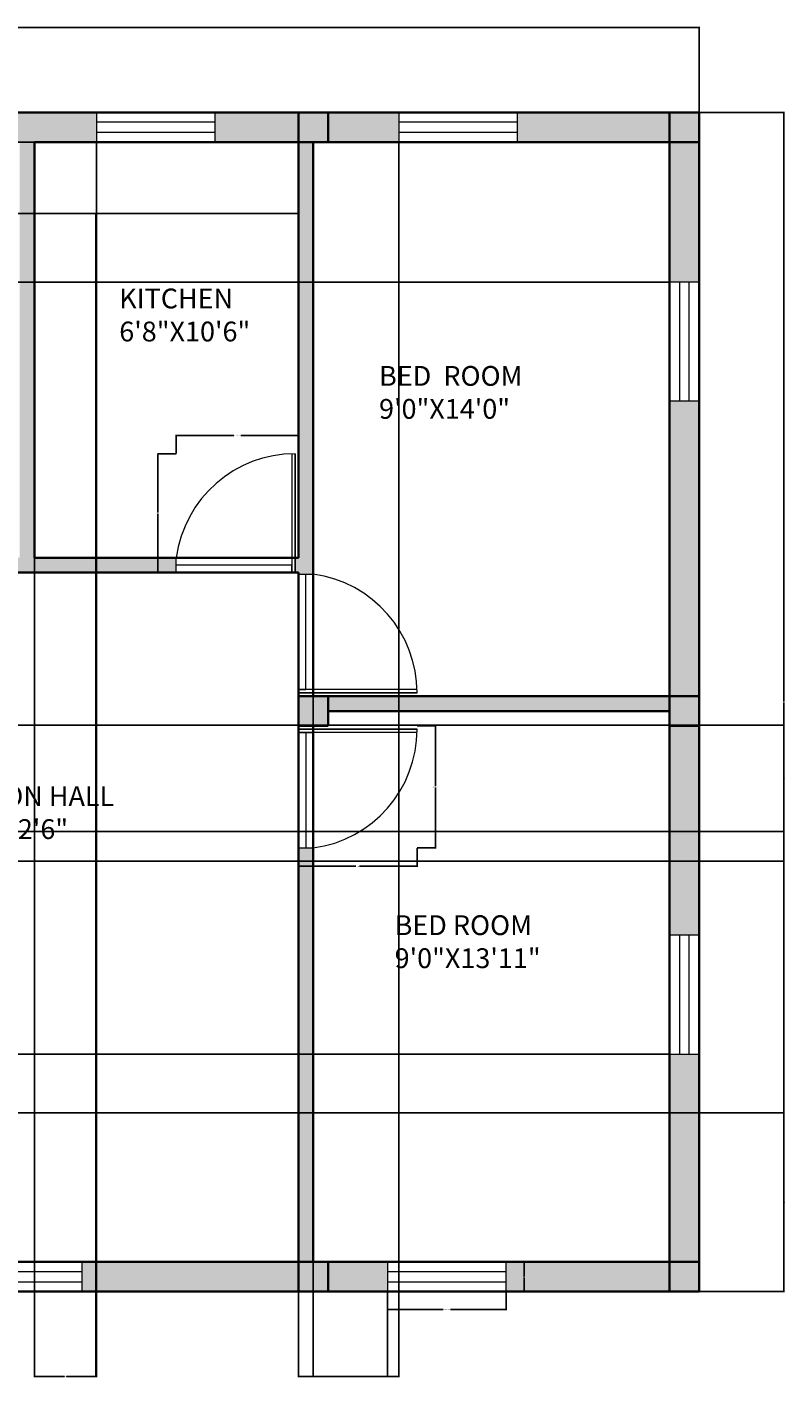
# Model space of a CAD drawing. Units: inches. Extents: x 6217 to 6782, y 16564 to 16973.
# Tile 3 of 3: x 6552 to 6782, y 16564 to 16973. Entities that reach past the tile are written whole.
import ezdxf

# ---------------------------------------------------------------- set-up
doc = ezdxf.new("R2010")
doc.units = ezdxf.units.IN
doc.header["$MEASUREMENT"] = 0
for name, color, linetype, lineweight in [('A-ANNO-DIMS', 2, 'Continuous', 18), ('A-AREA-IDEN', 7, 'Continuous', 18), ('A-COLS', 7, 'Continuous', 35), ('A-DOOR', 3, 'Continuous', 18), ('A-FLOR-FIXT', 8, 'Continuous', 25), ('A-GLAZ', 4, 'Continuous', 18), ('A-WALL', 7, 'Continuous', 35)]:
    doc.layers.add(name, color=color, linetype=linetype, lineweight=lineweight)
doc.layers.add('A-COLS-PATT', color=252, linetype='Continuous', lineweight=13, true_color=0x939598)
doc.layers.add('A-WALL-PATT', color=146, linetype='Continuous', lineweight=13, true_color=0x105689)
doc.styles.get("Standard").update_dxf_attribs({"font": 'arial.ttf'})
doc.dimstyles.get("Standard").update_dxf_attribs({"dimtxt": 0.18, "dimasz": 0.18, "dimexe": 0.18, "dimexo": 0.0625, "dimgap": 0.09, "dimtad": 0, "dimtih": 1, "dimtoh": 1, "dimdec": 4, "dimzin": 0, "dimdsep": 46, "dimtxsty": 'Standard', "dimcen": 0.09, "dimadec": 0, "dimazin": 0, "dimtfac": 1, "dimtdec": 4, "dimtofl": 0, "dimtmove": 0, "dimatfit": 3, "dimfxl": 1, "dimtolj": 1, "dimtzin": 0, "dimarcsym": 0})

# ---------------------------------------------------------------- blocks, each defined once
blk = doc.blocks.new('WIN-36')
for p, q in [((0, 9), (0, 0)), ((36, 9), (0, 9)), ((36, 0), (36, 9)), ((36, 6), (0, 6)), ((0, 3), (36, 3)), ((0, 0), (36, 0))]:
    blk.add_line(p, q)
blk = doc.blocks.new('DOOR-SINGLE-36-A')
for p, q in [((0, 36), (-4.5, 36)), ((-2.25, 1), (-2.25, 36)), ((0, 0), (0, 36)), ((-36, 1), (0, 1)), ((0, 0), (-36, 0)), ((-36, 0), (0, 0)), ((0, 1), (-4.5, 1)), ((-4.5, 1), (-2.25, 1)), ((0, -1), (0, 0))]:
    blk.add_line(p, q)
blk.add_arc((0.32, 0), 36.32, 97.6281, 180)
blk = doc.blocks.new('DOOR-SINGLE-36-B')
for p, q in [((-1, 36), (-1, 0)), ((0, 0), (0, 36)), ((0, 36), (0, 0)), ((-36, 0), (-36, 4.5)), ((-1, 4.5), (-1, 0)), ((-1, 2.25), (-36, 2.25)), ((0, 0), (-36, 0)), ((-1, 0), (-1, 2.25)), ((1, 0), (0, 0))]:
    blk.add_line(p, q)
blk.add_arc((0, -0.32), 36.32, 90, 172.3719)
blk = doc.blocks.new('*D6')
at = {"layer": 'A-ANNO-DIMS', "color": 0, "lineweight": -2, "transparency": 16777216}
for p, q in [((6661.06, 16589.44), (6661.06, 16583.92)), ((6697.06, 16589.44), (6697.06, 16583.92)), ((6661.24, 16584.1), (6677.95, 16584.1)), ((6696.88, 16584.1), (6680.18, 16584.1))]:
    blk.add_line(p, q, dxfattribs=at)
at = {"layer": 'A-ANNO-DIMS', "color": 0, "transparency": 16777216}
for points in [[(6661.24, 16584.13), (6661.24, 16584.07), (6661.06, 16584.1)], [(6696.88, 16584.13), (6696.88, 16584.07), (6697.06, 16584.1)]]:
    blk.add_solid(points, dxfattribs=at)
at = {"layer": 'Defpoints', "color": 0, "transparency": 16777216}
for p in [(6661.06, 16589.5), (6697.06, 16589.5), (6697.06, 16584.1)]:
    blk.add_point(p, dxfattribs=at)
at = {"layer": 'A-ANNO-DIMS', "color": 0, "transparency": 16777216, "insert": (6679.06, 16584.1), "char_height": 0.18, "attachment_point": 5}
blk.add_mtext('\\A1;WINDOW 36 TYP.', dxfattribs=at)
blk = doc.blocks.new('*D7')
at = {"layer": 'A-ANNO-DIMS', "color": 0, "lineweight": -2, "transparency": 16777216}
for p, q in [((6697.13, 16598.5), (6702.64, 16598.5)), ((6702.46, 16598.32), (6702.46, 16594.19)), ((6702.46, 16589.68), (6702.46, 16593.82)), ((6697.13, 16589.5), (6702.64, 16589.5))]:
    blk.add_line(p, q, dxfattribs=at)
at = {"layer": 'A-ANNO-DIMS', "color": 0, "transparency": 16777216}
for points in [[(6702.43, 16598.32), (6702.49, 16598.32), (6702.46, 16598.5)], [(6702.43, 16589.68), (6702.49, 16589.68), (6702.46, 16589.5)]]:
    blk.add_solid(points, dxfattribs=at)
at = {"layer": 'Defpoints', "color": 0, "transparency": 16777216}
for p in [(6697.06, 16598.5), (6702.46, 16598.5), (6697.06, 16589.5)]:
    blk.add_point(p, dxfattribs=at)
at = {"layer": 'A-ANNO-DIMS', "color": 0, "transparency": 16777216, "insert": (6702.46, 16594), "char_height": 0.18, "attachment_point": 5}
blk.add_mtext('\\A1;9 TYP.', dxfattribs=at)
blk = doc.blocks.new('*D10')
at = {"layer": 'A-ANNO-DIMS', "color": 0, "lineweight": -2, "transparency": 16777216}
for p, q in [((6670.09, 16761), (6675.76, 16761)), ((6675.58, 16760.82), (6675.58, 16742.69)), ((6675.58, 16724.18), (6675.58, 16742.32)), ((6670.09, 16724), (6675.76, 16724))]:
    blk.add_line(p, q, dxfattribs=at)
at = {"layer": 'A-ANNO-DIMS', "color": 0, "transparency": 16777216}
for points in [[(6675.55, 16760.82), (6675.61, 16760.82), (6675.58, 16761)], [(6675.55, 16724.18), (6675.61, 16724.18), (6675.58, 16724)]]:
    blk.add_solid(points, dxfattribs=at)
at = {"layer": 'Defpoints', "color": 0, "transparency": 16777216}
for p in [(6670.03, 16761), (6670.03, 16724), (6675.58, 16724)]:
    blk.add_point(p, dxfattribs=at)
at = {"layer": 'A-ANNO-DIMS', "color": 0, "transparency": 16777216, "insert": (6675.58, 16742.5), "char_height": 0.18, "attachment_point": 5}
blk.add_mtext('\\A1;DOOR A 37 TYP.', dxfattribs=at)
blk = doc.blocks.new('*D11')
at = {"layer": 'A-ANNO-DIMS', "color": 0, "lineweight": -2, "transparency": 16777216}
for p, q in [((6634.03, 16723.94), (6634.03, 16718.27)), ((6670.03, 16723.94), (6670.03, 16718.27)), ((6634.21, 16718.45), (6651.5, 16718.45)), ((6669.85, 16718.45), (6652.56, 16718.45))]:
    blk.add_line(p, q, dxfattribs=at)
at = {"layer": 'A-ANNO-DIMS', "color": 0, "transparency": 16777216}
for points in [[(6634.21, 16718.48), (6634.21, 16718.42), (6634.03, 16718.45)], [(6669.85, 16718.48), (6669.85, 16718.42), (6670.03, 16718.45)]]:
    blk.add_solid(points, dxfattribs=at)
at = {"layer": 'Defpoints', "color": 0, "transparency": 16777216}
for p in [(6634.03, 16724), (6670.03, 16724), (6634.03, 16718.45)]:
    blk.add_point(p, dxfattribs=at)
at = {"layer": 'A-ANNO-DIMS', "color": 0, "transparency": 16777216, "insert": (6652.03, 16718.45), "char_height": 0.18, "attachment_point": 5}
blk.add_mtext('\\A1;36 TYP.', dxfattribs=at)
blk = doc.blocks.new('*D12')
at = {"layer": 'A-ANNO-DIMS', "color": 0, "lineweight": -2, "transparency": 16777216}
for p, q in [((6597.03, 16843.57), (6597.03, 16849.23)), ((6597.21, 16849.05), (6614.47, 16849.05)), ((6633.85, 16849.05), (6616.58, 16849.05)), ((6634.03, 16843.57), (6634.03, 16849.23))]:
    blk.add_line(p, q, dxfattribs=at)
at = {"layer": 'A-ANNO-DIMS', "color": 0, "transparency": 16777216}
for points in [[(6597.21, 16849.08), (6597.21, 16849.02), (6597.03, 16849.05)], [(6633.85, 16849.08), (6633.85, 16849.02), (6634.03, 16849.05)]]:
    blk.add_solid(points, dxfattribs=at)
at = {"layer": 'Defpoints', "color": 0, "transparency": 16777216}
for p in [(6634.03, 16849.05), (6597.03, 16843.5), (6634.03, 16843.5)]:
    blk.add_point(p, dxfattribs=at)
at = {"layer": 'A-ANNO-DIMS', "color": 0, "transparency": 16777216, "insert": (6615.53, 16849.05), "char_height": 0.18, "attachment_point": 5}
blk.add_mtext('\\A1;DOOR B 37 TYP.', dxfattribs=at)
blk = doc.blocks.new('*D13')
at = {"layer": 'A-ANNO-DIMS', "color": 0, "lineweight": -2, "transparency": 16777216}
for p, q in [((6596.97, 16843.5), (6591.3, 16843.5)), ((6591.48, 16843.32), (6591.48, 16825.69)), ((6591.48, 16807.68), (6591.48, 16825.32)), ((6596.97, 16807.5), (6591.3, 16807.5))]:
    blk.add_line(p, q, dxfattribs=at)
at = {"layer": 'A-ANNO-DIMS', "color": 0, "transparency": 16777216}
for points in [[(6591.45, 16843.32), (6591.51, 16843.32), (6591.48, 16843.5)], [(6591.45, 16807.68), (6591.51, 16807.68), (6591.48, 16807.5)]]:
    blk.add_solid(points, dxfattribs=at)
at = {"layer": 'Defpoints', "color": 0, "transparency": 16777216}
for p in [(6591.48, 16843.5), (6597.03, 16843.5), (6597.03, 16807.5)]:
    blk.add_point(p, dxfattribs=at)
at = {"layer": 'A-ANNO-DIMS', "color": 0, "transparency": 16777216, "insert": (6591.48, 16825.5), "char_height": 0.18, "attachment_point": 5}
blk.add_mtext('\\A1;36 TYP.', dxfattribs=at)
blk = doc.blocks.new('*D16')
at = {"layer": 'A-ANNO-DIMS', "color": 0, "lineweight": -2, "transparency": 16777216}
for p, q in [((6243.53, 16812.07), (6243.53, 16972.89)), ((6243.71, 16972.71), (6499.24, 16972.71)), ((6755.35, 16972.71), (6499.82, 16972.71)), ((6755.53, 16947.07), (6755.53, 16972.89))]:
    blk.add_line(p, q, dxfattribs=at)
at = {"layer": 'A-ANNO-DIMS', "color": 0, "transparency": 16777216}
for points in [[(6243.71, 16972.74), (6243.71, 16972.68), (6243.53, 16972.71)], [(6755.35, 16972.74), (6755.35, 16972.68), (6755.53, 16972.71)]]:
    blk.add_solid(points, dxfattribs=at)
at = {"layer": 'Defpoints', "color": 0, "transparency": 16777216}
for p in [(6755.53, 16972.71), (6755.53, 16947), (6243.53, 16812)]:
    blk.add_point(p, dxfattribs=at)
at = {"layer": 'A-ANNO-DIMS', "color": 0, "transparency": 16777216, "insert": (6499.53, 16972.71), "char_height": 0.18, "attachment_point": 5}
blk.add_mtext('\\A1;512', dxfattribs=at)
blk = doc.blocks.new('*D17')
at = {"layer": 'A-ANNO-DIMS', "color": 0, "lineweight": -2, "transparency": 16777216}
for p, q in [((6755.59, 16947), (6781.41, 16947)), ((6781.23, 16946.82), (6781.23, 16768.44)), ((6781.23, 16589.68), (6781.23, 16768.07)), ((6755.59, 16589.5), (6781.41, 16589.5))]:
    blk.add_line(p, q, dxfattribs=at)
at = {"layer": 'A-ANNO-DIMS', "color": 0, "transparency": 16777216}
for points in [[(6781.2, 16946.82), (6781.26, 16946.82), (6781.23, 16947)], [(6781.2, 16589.68), (6781.26, 16589.68), (6781.23, 16589.5)]]:
    blk.add_solid(points, dxfattribs=at)
at = {"layer": 'Defpoints', "color": 0, "transparency": 16777216}
for p in [(6755.53, 16947), (6781.23, 16947), (6755.53, 16589.5)]:
    blk.add_point(p, dxfattribs=at)
at = {"layer": 'A-ANNO-DIMS', "color": 0, "transparency": 16777216, "insert": (6781.23, 16768.25), "char_height": 0.18, "attachment_point": 5}
blk.add_mtext('\\A1;357.5', dxfattribs=at)
blk = doc.blocks.new('*D24')
at = {"layer": 'A-ANNO-DIMS', "color": 0, "lineweight": -2, "transparency": 16777216}
for p, q in [((6554.03, 16937.94), (6554.03, 16563.62)), ((6572.83, 16937.94), (6572.83, 16563.62)), ((6554.21, 16563.8), (6563.11, 16563.8)), ((6572.65, 16563.8), (6563.74, 16563.8))]:
    blk.add_line(p, q, dxfattribs=at)
at = {"layer": 'A-ANNO-DIMS', "color": 0, "transparency": 16777216}
for points in [[(6554.21, 16563.83), (6554.21, 16563.77), (6554.03, 16563.8)], [(6572.65, 16563.83), (6572.65, 16563.77), (6572.83, 16563.8)]]:
    blk.add_solid(points, dxfattribs=at)
at = {"layer": 'Defpoints', "color": 0, "transparency": 16777216}
for p in [(6554.03, 16938), (6572.83, 16938), (6572.83, 16563.8)]:
    blk.add_point(p, dxfattribs=at)
at = {"layer": 'A-ANNO-DIMS', "color": 0, "transparency": 16777216, "insert": (6563.43, 16563.8), "char_height": 0.18, "attachment_point": 5}
blk.add_mtext('\\A1;18.8', dxfattribs=at)
blk = doc.blocks.new('*D25')
at = {"layer": 'A-ANNO-DIMS', "color": 0, "lineweight": -2, "transparency": 16777216}
for p, q in [((6638.53, 16937.94), (6638.53, 16563.62)), ((6664.44, 16937.94), (6664.44, 16563.62)), ((6638.71, 16563.8), (6651.11, 16563.8)), ((6664.26, 16563.8), (6651.86, 16563.8))]:
    blk.add_line(p, q, dxfattribs=at)
at = {"layer": 'A-ANNO-DIMS', "color": 0, "transparency": 16777216}
for points in [[(6638.71, 16563.83), (6638.71, 16563.77), (6638.53, 16563.8)], [(6664.26, 16563.83), (6664.26, 16563.77), (6664.44, 16563.8)]]:
    blk.add_solid(points, dxfattribs=at)
at = {"layer": 'Defpoints', "color": 0, "transparency": 16777216}
for p in [(6638.53, 16938), (6664.44, 16938), (6664.44, 16563.8)]:
    blk.add_point(p, dxfattribs=at)
at = {"layer": 'A-ANNO-DIMS', "color": 0, "transparency": 16777216, "insert": (6651.48, 16563.8), "char_height": 0.18, "attachment_point": 5}
blk.add_mtext('\\A1;25.91', dxfattribs=at)
blk = doc.blocks.new('*D26')
at = {"layer": 'A-ANNO-DIMS', "color": 0, "lineweight": -2, "transparency": 16777216}
for p, q in [((6755.47, 16938), (6217.65, 16938)), ((6217.83, 16937.82), (6217.83, 16916.95)), ((6217.83, 16895.7), (6217.83, 16916.58)), ((6746.47, 16895.52), (6217.65, 16895.52))]:
    blk.add_line(p, q, dxfattribs=at)
at = {"layer": 'A-ANNO-DIMS', "color": 0, "transparency": 16777216}
for points in [[(6217.8, 16937.82), (6217.86, 16937.82), (6217.83, 16938)], [(6217.8, 16895.7), (6217.86, 16895.7), (6217.83, 16895.52)]]:
    blk.add_solid(points, dxfattribs=at)
at = {"layer": 'Defpoints', "color": 0, "transparency": 16777216}
for p in [(6755.53, 16938), (6217.83, 16895.52), (6746.53, 16895.52)]:
    blk.add_point(p, dxfattribs=at)
at = {"layer": 'A-ANNO-DIMS', "color": 0, "transparency": 16777216, "insert": (6217.83, 16916.76), "char_height": 0.18, "attachment_point": 5}
blk.add_mtext('\\A1;42.48', dxfattribs=at)
blk = doc.blocks.new('*D27')
at = {"layer": 'A-ANNO-DIMS', "color": 0, "lineweight": -2, "transparency": 16777216}
for p, q in [((6746.47, 16661.53), (6217.65, 16661.53)), ((6217.83, 16661.35), (6217.83, 16625.7)), ((6217.83, 16589.68), (6217.83, 16625.33)), ((6746.47, 16589.5), (6217.65, 16589.5))]:
    blk.add_line(p, q, dxfattribs=at)
at = {"layer": 'A-ANNO-DIMS', "color": 0, "transparency": 16777216}
for points in [[(6217.8, 16661.35), (6217.86, 16661.35), (6217.83, 16661.53)], [(6217.8, 16589.68), (6217.86, 16589.68), (6217.83, 16589.5)]]:
    blk.add_solid(points, dxfattribs=at)
at = {"layer": 'Defpoints', "color": 0, "transparency": 16777216}
for p in [(6217.83, 16661.53), (6746.53, 16661.53), (6746.53, 16589.5)]:
    blk.add_point(p, dxfattribs=at)
at = {"layer": 'A-ANNO-DIMS', "color": 0, "transparency": 16777216, "insert": (6217.83, 16625.52), "char_height": 0.18, "attachment_point": 5}
blk.add_mtext('\\A1;72.03', dxfattribs=at)
blk = doc.blocks.new('*D28')
at = {"layer": 'A-ANNO-DIMS', "color": 0, "lineweight": -2, "transparency": 16777216}
for p, q in [((6288.59, 16643.72), (6781.41, 16643.72)), ((6781.23, 16643.54), (6781.23, 16616.79)), ((6781.23, 16589.68), (6781.23, 16616.43)), ((6288.59, 16589.5), (6781.41, 16589.5))]:
    blk.add_line(p, q, dxfattribs=at)
at = {"layer": 'A-ANNO-DIMS', "color": 0, "transparency": 16777216}
for points in [[(6781.2, 16643.54), (6781.26, 16643.54), (6781.23, 16643.72)], [(6781.2, 16589.68), (6781.26, 16589.68), (6781.23, 16589.5)]]:
    blk.add_solid(points, dxfattribs=at)
at = {"layer": 'Defpoints', "color": 0, "transparency": 16777216}
for p in [(6288.53, 16643.72), (6781.23, 16643.72), (6288.53, 16589.5)]:
    blk.add_point(p, dxfattribs=at)
at = {"layer": 'A-ANNO-DIMS', "color": 0, "transparency": 16777216, "insert": (6781.23, 16616.61), "char_height": 0.18, "attachment_point": 5}
blk.add_mtext('\\A1;54.22', dxfattribs=at)
blk = doc.blocks.new('*D32')
at = {"layer": 'A-ANNO-DIMS', "color": 0, "lineweight": -2, "transparency": 16777216}
for p, q in [((6634.03, 16589.44), (6634.03, 16563.62)), ((6661.06, 16589.44), (6661.06, 16563.62)), ((6634.21, 16563.8), (6647.08, 16563.8)), ((6660.88, 16563.8), (6648.01, 16563.8))]:
    blk.add_line(p, q, dxfattribs=at)
at = {"layer": 'A-ANNO-DIMS', "color": 0, "transparency": 16777216}
for points in [[(6634.21, 16563.83), (6634.21, 16563.77), (6634.03, 16563.8)], [(6660.88, 16563.83), (6660.88, 16563.77), (6661.06, 16563.8)]]:
    blk.add_solid(points, dxfattribs=at)
at = {"layer": 'Defpoints', "color": 0, "transparency": 16777216}
for p in [(6634.03, 16589.5), (6661.06, 16589.5), (6661.06, 16563.8)]:
    blk.add_point(p, dxfattribs=at)
at = {"layer": 'A-ANNO-DIMS', "color": 0, "transparency": 16777216, "insert": (6647.55, 16563.8), "char_height": 0.18, "attachment_point": 5}
blk.add_mtext('\\A1;27.036', dxfattribs=at)
blk = doc.blocks.new('*D35')
at = {"layer": 'A-ANNO-DIMS', "color": 0, "lineweight": -2, "transparency": 16777216}
for p, q in [((6431.24, 16761.25), (6781.41, 16761.25)), ((6781.23, 16761.07), (6781.23, 16745.31)), ((6781.23, 16729.18), (6781.23, 16744.95)), ((6431.24, 16729), (6781.41, 16729))]:
    blk.add_line(p, q, dxfattribs=at)
at = {"layer": 'A-ANNO-DIMS', "color": 0, "transparency": 16777216}
for points in [[(6781.2, 16761.07), (6781.26, 16761.07), (6781.23, 16761.25)], [(6781.2, 16729.18), (6781.26, 16729.18), (6781.23, 16729)]]:
    blk.add_solid(points, dxfattribs=at)
at = {"layer": 'Defpoints', "color": 0, "transparency": 16777216}
for p in [(6431.17, 16761.25), (6781.23, 16761.25), (6431.17, 16729)]:
    blk.add_point(p, dxfattribs=at)
at = {"layer": 'A-ANNO-DIMS', "color": 0, "transparency": 16777216, "insert": (6781.23, 16745.13), "char_height": 0.18, "attachment_point": 5}
blk.add_mtext('\\A1;32.25', dxfattribs=at)
blk = doc.blocks.new('*D38')
at = {"layer": 'A-ANNO-DIMS', "color": 0, "lineweight": -2, "transparency": 16777216}
for p, q in [((6554.03, 16937.94), (6554.03, 16563.62)), ((6572.66, 16916.23), (6572.66, 16563.62)), ((6554.21, 16563.8), (6562.89, 16563.8)), ((6572.48, 16563.8), (6563.8, 16563.8))]:
    blk.add_line(p, q, dxfattribs=at)
at = {"layer": 'A-ANNO-DIMS', "color": 0, "transparency": 16777216}
for points in [[(6554.21, 16563.83), (6554.21, 16563.77), (6554.03, 16563.8)], [(6572.48, 16563.83), (6572.48, 16563.77), (6572.66, 16563.8)]]:
    blk.add_solid(points, dxfattribs=at)
at = {"layer": 'Defpoints', "color": 0, "transparency": 16777216}
for p in [(6554.03, 16938), (6572.66, 16916.3), (6554.03, 16563.8)]:
    blk.add_point(p, dxfattribs=at)
at = {"layer": 'A-ANNO-DIMS', "color": 0, "transparency": 16777216, "insert": (6563.34, 16563.8), "char_height": 0.18, "attachment_point": 5}
blk.add_mtext('\\A1;18.627', dxfattribs=at)
blk = doc.blocks.new('*D39')
at = {"layer": 'A-ANNO-DIMS', "color": 0, "lineweight": -2, "transparency": 16777216}
for p, q in [((6633.97, 16938), (6217.65, 16938)), ((6217.83, 16937.82), (6217.83, 16927.33)), ((6217.83, 16916.48), (6217.83, 16926.97)), ((6633.97, 16916.3), (6217.65, 16916.3))]:
    blk.add_line(p, q, dxfattribs=at)
at = {"layer": 'A-ANNO-DIMS', "color": 0, "transparency": 16777216}
for points in [[(6217.8, 16937.82), (6217.86, 16937.82), (6217.83, 16938)], [(6217.8, 16916.48), (6217.86, 16916.48), (6217.83, 16916.3)]]:
    blk.add_solid(points, dxfattribs=at)
at = {"layer": 'Defpoints', "color": 0, "transparency": 16777216}
for p in [(6217.83, 16938), (6634.03, 16938), (6634.03, 16916.3)]:
    blk.add_point(p, dxfattribs=at)
at = {"layer": 'A-ANNO-DIMS', "color": 0, "transparency": 16777216, "insert": (6217.83, 16927.15), "char_height": 0.18, "attachment_point": 5}
blk.add_mtext('\\A1;21.706', dxfattribs=at)
blk = doc.blocks.new('*D42')
at = {"layer": 'A-ANNO-DIMS', "color": 0, "lineweight": -2, "transparency": 16777216}
for p, q in [((6472.09, 16729), (6781.41, 16729)), ((6781.23, 16728.82), (6781.23, 16724.69)), ((6781.23, 16720.18), (6781.23, 16724.32)), ((6472.09, 16720), (6781.41, 16720))]:
    blk.add_line(p, q, dxfattribs=at)
at = {"layer": 'A-ANNO-DIMS', "color": 0, "transparency": 16777216}
for points in [[(6781.2, 16728.82), (6781.26, 16728.82), (6781.23, 16729)], [(6781.2, 16720.18), (6781.26, 16720.18), (6781.23, 16720)]]:
    blk.add_solid(points, dxfattribs=at)
at = {"layer": 'Defpoints', "color": 0, "transparency": 16777216}
for p in [(6472.03, 16729), (6781.23, 16729), (6472.03, 16720)]:
    blk.add_point(p, dxfattribs=at)
at = {"layer": 'A-ANNO-DIMS', "color": 0, "transparency": 16777216, "insert": (6781.23, 16724.5), "char_height": 0.18, "attachment_point": 5}
blk.add_mtext('\\A1;9', dxfattribs=at)

msp = doc.modelspace()

# ---------------------------------------------------------------- hatches: boundary and pattern name
at = {"layer": 'A-COLS-PATT'}
h = msp.add_hatch(color=256, dxfattribs=at)
h.dxf.hatch_style = 1
h.paths.add_polyline_path([(6288.5285, 16947.0033), (6279.5285, 16947.0033), (6279.5285, 16938.0033), (6288.5285, 16938.0033)])
h.paths.add_polyline_path([(6449.0285, 16947.0033), (6440.0285, 16947.0033), (6440.0285, 16938.0033), (6449.0285, 16938.0033)])
h.paths.add_polyline_path([(6506.0285, 16947.0033), (6497.0285, 16947.0033), (6497.0285, 16938.0033), (6506.0285, 16938.0033)])
h.paths.add_polyline_path([(6643.0285, 16947.0033), (6634.0285, 16947.0033), (6634.0285, 16938.0033), (6643.0285, 16938.0033)])
h.paths.add_polyline_path([(6755.5285, 16947.0033), (6746.5285, 16947.0033), (6746.5285, 16938.0033), (6755.5285, 16938.0033)])
h.paths.add_polyline_path([(6755.5285, 16770.0033), (6746.5285, 16770.0033), (6746.5285, 16761.0033), (6755.5285, 16761.0033)])
h.paths.add_polyline_path([(6643.0285, 16770.0033), (6634.0285, 16770.0033), (6634.0285, 16761.0033), (6643.0285, 16761.0033)])
h.paths.add_polyline_path([(6755.5285, 16598.5033), (6746.5285, 16598.5033), (6746.5285, 16589.5033), (6755.5285, 16589.5033)])
h.paths.add_polyline_path([(6643.0285, 16598.5033), (6634.0285, 16598.5033), (6634.0285, 16589.5033), (6643.0285, 16589.5033)])
h.paths.add_polyline_path([(6517.0285, 16598.5033), (6508.0285, 16598.5033), (6508.0285, 16589.5033), (6517.0285, 16589.5033)])
h.paths.add_polyline_path([(6472.0285, 16598.5033), (6463.0285, 16598.5033), (6463.0285, 16589.5033), (6472.0285, 16589.5033)])
h.paths.add_polyline_path([(6472.0285, 16729.0033), (6463.0285, 16729.0033), (6463.0285, 16720.0033), (6472.0285, 16720.0033)])
h.paths.add_polyline_path([(6288.5285, 16598.5033), (6279.5285, 16598.5033), (6279.5285, 16589.5033), (6288.5285, 16589.5033)])
h.paths.add_polyline_path([(6288.5285, 16729.0033), (6279.5285, 16729.0033), (6279.5285, 16720.0033), (6288.5285, 16720.0033)])
h.paths.add_polyline_path([(6288.5285, 16812.0033), (6279.5285, 16812.0033), (6279.5285, 16803.0033), (6288.5285, 16803.0033)])
h.paths.add_polyline_path([(6449.0285, 16812.0033), (6440.0285, 16812.0033), (6440.0285, 16803.0033), (6449.0285, 16803.0033)])
at = {"layer": 'A-WALL-PATT'}
h = msp.add_hatch(color=256, dxfattribs=at)
h.dxf.hatch_style = 1
h.paths.add_polyline_path([(6497.0285, 16947.0033), (6484.6293, 16947.0033), (6484.6293, 16938.0033), (6497.0285, 16938.0033)])
h.paths.add_polyline_path([(6513.3814, 16947.0033), (6506.0285, 16947.0033), (6506.0285, 16938.0033), (6513.3814, 16938.0033)])
h.paths.add_polyline_path([(6572.828, 16947.0033), (6537.3814, 16947.0033), (6537.3814, 16938.0033), (6549.5285, 16938.0033), (6549.5285, 16812.0033), (6534.5285, 16812.0033), (6534.5285, 16807.5033), (6597.0285, 16807.5033), (6597.0285, 16812.0033), (6554.0285, 16812.0033), (6554.0285, 16938.0033), (6572.828, 16938.0033)])
h.paths.add_polyline_path([(6501.5285, 16938.0033), (6497.0285, 16938.0033), (6497.0285, 16854.0033), (6449.0285, 16854.0033), (6449.0285, 16855.0033), (6444.5285, 16855.0033), (6444.5285, 16854.0033), (6444.5285, 16849.0033), (6449.0285, 16849.0033), (6449.0285, 16849.5033), (6497.0285, 16849.5033), (6497.0285, 16807.5033), (6502.5285, 16807.5033), (6502.5285, 16812.0033), (6501.5285, 16812.0033)])
h.paths.add_polyline_path([(6634.0285, 16947.0033), (6608.828, 16947.0033), (6608.828, 16938.0033), (6634.0285, 16938.0033)])
h.paths.add_polyline_path([(6664.4385, 16947.0033), (6643.0285, 16947.0033), (6643.0285, 16938.0033), (6664.4385, 16938.0033)])
h.paths.add_polyline_path([(6638.5285, 16938.0033), (6634.0285, 16938.0033), (6634.0285, 16812.0033), (6633.0285, 16812.0033), (6633.0285, 16807.5033), (6634.0285, 16807.5033), (6634.0285, 16807.0033), (6638.5285, 16807.0033)])
h.paths.add_polyline_path([(6746.5285, 16947.0033), (6700.4385, 16947.0033), (6700.4385, 16938.0033), (6746.5285, 16938.0033)])
h.paths.add_polyline_path([(6755.5285, 16938.0033), (6746.5285, 16938.0033), (6746.5285, 16895.525), (6755.5285, 16895.525)])
h.paths.add_polyline_path([(6755.5285, 16859.525), (6746.5285, 16859.525), (6746.5285, 16770.0033), (6755.5285, 16770.0033)])
h.paths.add_polyline_path([(6746.5285, 16770.0033), (6643.0285, 16770.0033), (6643.0285, 16765.5033), (6746.5285, 16765.5033)])
h.paths.add_polyline_path([(6755.5285, 16761.0033), (6746.5285, 16761.0033), (6746.5285, 16697.5292), (6755.5285, 16697.5292)])
h.paths.add_polyline_path([(6440.0285, 16812.0033), (6288.5285, 16812.0033), (6288.5285, 16807.5033), (6440.0285, 16807.5033)])
h.paths.add_polyline_path([(6288.5285, 16938.0033), (6279.5285, 16938.0033), (6279.5285, 16849.0033), (6288.5285, 16849.0033)])
h.paths.add_polyline_path([(6279.5285, 16729.0033), (6248.0285, 16729.0033), (6248.0285, 16807.5033), (6279.5285, 16807.5033), (6279.5285, 16812.0033), (6243.5285, 16812.0033), (6243.5285, 16724.5033), (6279.5285, 16724.5033)])
h.paths.add_polyline_path([(6463.0285, 16729.0033), (6288.5285, 16729.0033), (6288.5285, 16724.5033), (6463.0285, 16724.5033)])
h.paths.add_polyline_path([(6288.5285, 16720.0033), (6279.5285, 16720.0033), (6279.5285, 16679.7207), (6288.5285, 16679.7207)])
h.paths.add_polyline_path([(6288.5285, 16643.7207), (6279.5285, 16643.7207), (6279.5285, 16598.5033), (6288.5285, 16598.5033)])
h.paths.add_polyline_path([(6350.2697, 16598.5033), (6288.5285, 16598.5033), (6288.5285, 16589.5033), (6350.2697, 16589.5033)])
h.paths.add_polyline_path([(6463.0285, 16598.5033), (6386.2697, 16598.5033), (6386.2697, 16589.5033), (6463.0285, 16589.5033)])
h.paths.add_polyline_path([(6472.0285, 16683.0033), (6467.5285, 16683.0033), (6467.5285, 16598.5033), (6472.0285, 16598.5033)])
h.paths.add_polyline_path([(6532.5191, 16598.5033), (6517.0285, 16598.5033), (6517.0285, 16589.5033), (6532.5191, 16589.5033)])
h.paths.add_polyline_path([(6634.0285, 16598.5033), (6568.5191, 16598.5033), (6568.5191, 16589.5033), (6634.0285, 16589.5033)])
h.paths.add_polyline_path([(6661.0648, 16598.5033), (6643.0285, 16598.5033), (6643.0285, 16589.5033), (6661.0648, 16589.5033)])
h.paths.add_polyline_path([(6746.5285, 16598.5033), (6697.0648, 16598.5033), (6697.0648, 16589.5033), (6746.5285, 16589.5033)])
h.paths.add_polyline_path([(6755.5285, 16661.5292), (6746.5285, 16661.5292), (6746.5285, 16598.5033), (6755.5285, 16598.5033)])
h.paths.add_polyline_path([(6638.5285, 16724.0033), (6634.0285, 16724.0033), (6634.0285, 16598.5033), (6638.5285, 16598.5033)])

# ---------------------------------------------------------------- linework, layer by layer
at = {"layer": 'A-COLS'}
for p, q in [((6634.0285, 16947.0033), (6643.0285, 16947.0033)), ((6643.0285, 16947.0033), (6643.0285, 16938.0033)), ((6643.0285, 16938.0033), (6634.0285, 16938.0033)), ((6634.0285, 16770.0033), (6643.0285, 16770.0033)), ((6643.0285, 16770.0033), (6643.0285, 16761.0033)), ((6746.5285, 16770.0033), (6746.5285, 16761.0033)), ((6755.5285, 16761.0033), (6755.5285, 16770.0033)), ((6643.0285, 16761.0033), (6634.0285, 16761.0033)), ((6746.5285, 16761.0033), (6755.5285, 16761.0033)), ((6634.0285, 16598.5033), (6643.0285, 16598.5033)), ((6643.0285, 16598.5033), (6643.0285, 16589.5033))]:
    msp.add_line(p, q, dxfattribs=at)
at = {"layer": 'A-FLOR-FIXT'}
for p, q in [((6572.6559, 16812.0033), (6572.6559, 16916.2968)), ((6572.6559, 16916.2968), (6634.0285, 16916.2968))]:
    msp.add_line(p, q, dxfattribs=at)
at = {"layer": 'A-WALL'}
for p, q in [((6279.5285, 16947.0033), (6755.5285, 16947.0033)), ((6634.0285, 16947.0033), (6634.0285, 16812.0033)), ((6746.5285, 16947.0033), (6746.5285, 16589.5033)), ((6755.5285, 16947.0033), (6755.5285, 16589.5033)), ((6554.0285, 16938.0033), (6554.0285, 16812.0033)), ((6554.0285, 16938.0033), (6755.5285, 16938.0033)), ((6638.5285, 16938.0033), (6638.5285, 16770.0033)), ((6554.0285, 16812.0033), (6634.0285, 16812.0033)), ((6497.0285, 16807.5033), (6634.0285, 16807.5033)), ((6634.0285, 16807.5033), (6634.0285, 16589.5033)), ((6634.0285, 16770.0033), (6755.5285, 16770.0033)), ((6643.0285, 16765.5033), (6746.5285, 16765.5033)), ((6638.5285, 16761.0033), (6638.5285, 16598.5033)), ((6508.0285, 16598.5033), (6755.5285, 16598.5033)), ((6279.5285, 16589.5033), (6755.5285, 16589.5033))]:
    msp.add_line(p, q, dxfattribs=at)

# ---------------------------------------------------------------- block references
at = {"layer": 'A-DOOR'}
msp.add_blockref('DOOR-SINGLE-36-B', (6633.0285, 16807.5033), dxfattribs=at)
for name, p, rotation in [('DOOR-SINGLE-36-B', (6634.0285, 16771.0033), 269.9999999999954), ('DOOR-SINGLE-36-A', (6634.0285, 16760.0033), 180)]:
    msp.add_blockref(name, p, dxfattribs=dict(at, rotation=rotation))
at = {"layer": 'A-GLAZ'}
for p in [(6572.828, 16938.0033), (6664.4385, 16938.0033), (6532.5191, 16589.5033), (6661.0648, 16589.5033)]:
    msp.add_blockref('WIN-36', p, dxfattribs=at)
for p, rotation in [((6746.5285, 16895.525), 270.0000000000081), ((6746.5285, 16697.5292), 270.0000000000109)]:
    msp.add_blockref('WIN-36', p, dxfattribs=dict(at, rotation=rotation))

# ---------------------------------------------------------------- texts
at = {"layer": 'A-AREA-IDEN', "char_height": 6, "attachment_point": 1}
for s, width, insert in [('KITCHEN\\P6\'8"X10\'6"', 45.455487, (6579.7431, 16893.5753)), ('BED  ROOM\\P9\'0"X14\'0"', 64.386909, (6658.4865, 16870.1139)), ('COMMON HALL\\P13\'7"X12\'6"', 74.34141, (6519.987, 16742.7201)), ('BED ROOM\\P9\'0"X13\'11"', 59.878446, (6663.2128, 16703.5878))]:
    msp.add_mtext_dynamic_manual_height_columns(s, width=width, gutter_width=1, heights=[0], dxfattribs=dict(at, insert=insert))

# ---------------------------------------------------------------- dimensions: what is measured, and where the dimension line sits
at = {"layer": 'A-ANNO-DIMS'}
for base, p1, p2, override, picture, middle in [((6755.5285, 16972.7058), (6243.5285, 16812.0033), (6755.5285, 16947.0033), {"dimdec": 0, "dimlfac": 1, "dimrnd": 0, "dimzin": 0, "dimdsep": 46, "dimlunit": 2}, '*D16', (6499.5285, 16972.7058)), ((6572.828, 16563.8008), (6554.0285, 16938.0033), (6572.828, 16938.0033), {"dimdec": 1, "dimlfac": 1, "dimrnd": 0, "dimzin": 0, "dimdsep": 46, "dimlunit": 2}, '*D24', (6563.4282, 16563.8008)), ((6554.0285, 16563.8008), (6572.6559, 16916.2968), (6554.0285, 16938.0033), {"dimdec": 3, "dimlfac": 1, "dimrnd": 0, "dimzin": 0, "dimdsep": 46, "dimlunit": 2}, '*D38', (6563.3422, 16563.8008)), ((6664.4385, 16563.8008), (6638.5285, 16938.0033), (6664.4385, 16938.0033), {"dimdec": 2, "dimlfac": 1, "dimrnd": 0, "dimzin": 0, "dimdsep": 46, "dimlunit": 2}, '*D25', (6651.4835, 16563.8008)), ((6661.0648, 16563.8008), (6634.0285, 16589.5033), (6661.0648, 16589.5033), {"dimdec": 3, "dimlfac": 1, "dimrnd": 0, "dimzin": 0, "dimdsep": 46, "dimlunit": 2}, '*D32', (6647.5466, 16563.8008))]:
    dim = msp.add_linear_dim(base=base, p1=p1, p2=p2, dimstyle='Standard', override=override, dxfattribs=at)
    dim.commit()
    dim.dimension.update_dxf_attribs({"geometry": picture, "text_midpoint": middle})
for base, p1, p2, override, picture, middle in [((6781.231, 16947.0033), (6755.5285, 16589.5033), (6755.5285, 16947.0033), {"dimdec": 1, "dimlfac": 1, "dimrnd": 0, "dimzin": 0, "dimdsep": 46, "dimlunit": 2}, '*D17', (6781.231, 16768.2533)), ((6217.826, 16938.00326), (6634.0285, 16916.29685), (6634.0285, 16938.00326), {"dimdec": 3, "dimlfac": 1, "dimrnd": 0, "dimzin": 0, "dimdsep": 46, "dimlunit": 2}, '*D39', (6217.826, 16927.15005)), ((6217.826, 16895.525), (6755.5285, 16938.0033), (6746.5285, 16895.525), {"dimdec": 2, "dimlfac": 1, "dimrnd": 0, "dimzin": 0, "dimdsep": 46, "dimlunit": 2}, '*D26', (6217.826, 16916.7641)), ((6781.231, 16761.2533), (6431.174, 16729.0033), (6431.174, 16761.2533), {"dimdec": 2, "dimlfac": 1, "dimrnd": 0, "dimzin": 0, "dimdsep": 46, "dimlunit": 2}, '*D35', (6781.231, 16745.1283)), ((6781.231, 16729.0033), (6472.0285, 16720.0033), (6472.0285, 16729.0033), {"dimdec": 0, "dimlfac": 1, "dimrnd": 0, "dimzin": 0, "dimdsep": 46, "dimlunit": 2}, '*D42', (6781.231, 16724.5033)), ((6217.826, 16661.5292), (6746.5285, 16589.5033), (6746.5285, 16661.5292), {"dimdec": 2, "dimlfac": 1, "dimrnd": 0, "dimzin": 0, "dimdsep": 46, "dimlunit": 2}, '*D27', (6217.826, 16625.5162)), ((6781.231, 16643.7207), (6288.5285, 16589.5033), (6288.5285, 16643.7207), {"dimdec": 2, "dimlfac": 1, "dimrnd": 0, "dimzin": 0, "dimdsep": 46, "dimlunit": 2}, '*D28', (6781.231, 16616.612))]:
    dim = msp.add_linear_dim(base=base, p1=p1, p2=p2, angle=90, dimstyle='Standard', override=override, dxfattribs=at)
    dim.commit()
    dim.dimension.update_dxf_attribs({"geometry": picture, "text_midpoint": middle})
for base, p1, p2, text, picture, middle in [((6634.0285, 16849.0533), (6597.0285, 16843.5033), (6634.0285, 16843.5033), 'DOOR B <> TYP.', '*D12', (6615.5285, 16849.0533)), ((6697.0648, 16584.1033), (6661.0648, 16589.5033), (6697.0648, 16589.5033), 'WINDOW <> TYP.', '*D6', (6679.0648, 16584.1033))]:
    dim = msp.add_linear_dim(base=base, p1=p1, p2=p2, text=text, dimstyle='Standard', override={"dimdec": 0, "dimlfac": 1, "dimrnd": 0, "dimzin": 0, "dimdsep": 46, "dimlunit": 2}, dxfattribs=at)
    dim.commit()
    dim.dimension.update_dxf_attribs({"geometry": picture, "text_midpoint": middle})
for base, p1, p2, angle, text, picture, middle in [((6591.4785, 16843.5033), (6597.0285, 16807.5033), (6597.0285, 16843.5033), 90, '<> TYP.', '*D13', (6591.4785, 16825.5033)), ((6675.5785, 16724.0033), (6670.0285, 16761.0033), (6670.0285, 16724.0033), 270, 'DOOR A <> TYP.', '*D10', (6675.5785, 16742.5033)), ((6634.0285, 16718.4533), (6670.0285, 16724.0033), (6634.0285, 16724.0033), 180, '<> TYP.', '*D11', (6652.0285, 16718.4533)), ((6702.4648, 16598.5033), (6697.0648, 16589.5033), (6697.0648, 16598.5033), 90, '<> TYP.', '*D7', (6702.4648, 16594.0033))]:
    dim = msp.add_linear_dim(base=base, p1=p1, p2=p2, angle=angle, text=text, dimstyle='Standard', override={"dimdec": 0, "dimlfac": 1, "dimrnd": 0, "dimzin": 0, "dimdsep": 46, "dimlunit": 2}, dxfattribs=at)
    dim.commit()
    dim.dimension.update_dxf_attribs({"geometry": picture, "text_midpoint": middle})

doc.saveas('drawing.dxf')
